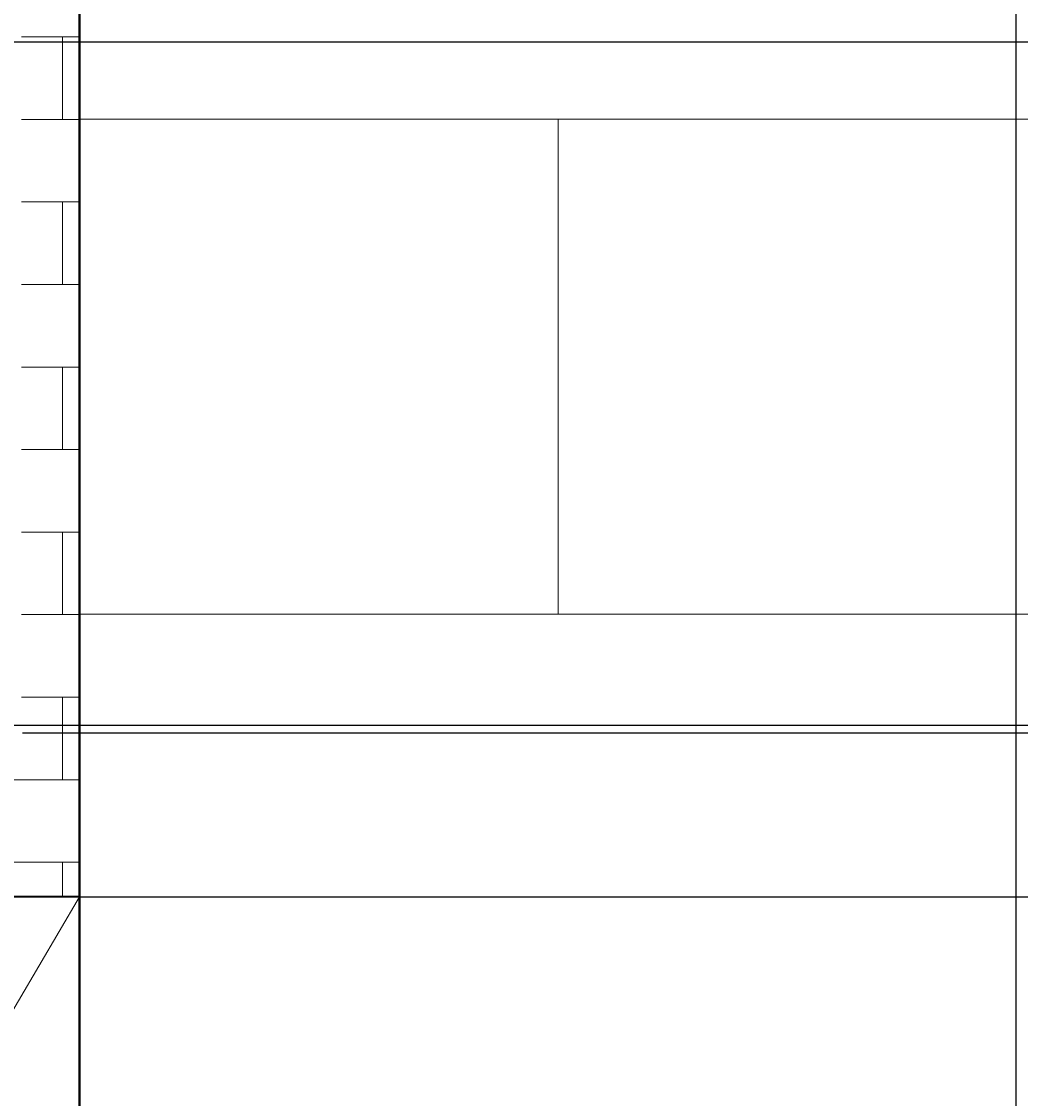
# Model space of a CAD drawing. Units: inches. Extents: x -26 to 776, y -22 to 650.
# Tile 19 of 62: x 285 to 358, y 145 to 223. Entities that reach past the tile are written whole.
import ezdxf

# ---------------------------------------------------------------- set-up
doc = ezdxf.new("R2010")
doc.units = ezdxf.units.IN
doc.header["$MEASUREMENT"] = 0
for name, color, linetype, lineweight in [('A-ANNO-DIMS', 2, 'Continuous', 18), ('A-WALL', 7, 'Continuous', 35), ('A-WALL-PATT', 8, 'Continuous', 13), ('A-WALL-TRIM', 7, 'Continuous', 18)]:
    doc.layers.add(name, color=color, linetype=linetype, lineweight=lineweight)
doc.styles.get("Standard").update_dxf_attribs({"font": 'arial.ttf'})
doc.dimstyles.get("Standard").update_dxf_attribs({"dimtxt": 0.5625, "dimasz": 0.18, "dimexe": 0.18, "dimexo": 0.0625, "dimgap": 0.09, "dimtad": 0, "dimtih": 1, "dimtoh": 1, "dimdec": 4, "dimzin": 0, "dimdsep": 46, "dimlunit": 4, "dimtxsty": 'Standard', "dimcen": 0.09, "dimadec": 0, "dimazin": 0, "dimtfac": 1, "dimtdec": 4, "dimtofl": 0, "dimtmove": 0, "dimatfit": 3, "dimfxl": 1, "dimtolj": 1, "dimtzin": 0, "dimarcsym": 0})

# ---------------------------------------------------------------- blocks, each defined once
blk = doc.blocks.new('*D26')
at = {"layer": 'A-ANNO-DIMS', "color": 0, "lineweight": -2, "transparency": 16777216}
for p, q in [((91.707, 171.973), (775.335, 171.973)), ((775.155, 171.793), (775.155, 166.105)), ((775.155, 159.662), (775.155, 165.351)), ((82.196, 159.482), (775.335, 159.482))]:
    blk.add_line(p, q, dxfattribs=at)
at = {"layer": 'A-ANNO-DIMS', "color": 0, "transparency": 16777216}
for points in [[(775.125, 171.793), (775.185, 171.793), (775.155, 171.973)], [(775.125, 159.662), (775.185, 159.662), (775.155, 159.482)]]:
    blk.add_solid(points, dxfattribs=at)
at = {"layer": 'Defpoints', "color": 0, "transparency": 16777216}
for p in [(91.645, 171.973), (775.155, 171.973), (82.134, 159.482)]:
    blk.add_point(p, dxfattribs=at)
at = {"layer": 'A-ANNO-DIMS', "color": 0, "transparency": 16777216, "insert": (775.155, 165.728), "char_height": 0.5625, "attachment_point": 5}
blk.add_mtext('\\A1;12.49', dxfattribs=at)
blk = doc.blocks.new('*D28')
at = {"layer": 'A-ANNO-DIMS', "color": 0, "lineweight": -2, "transparency": 16777216}
for p, q in [((285.08, 314.119), (775.335, 314.119)), ((775.155, 313.939), (775.155, 243.141)), ((775.155, 171.597), (775.155, 242.396)), ((285.08, 171.417), (775.335, 171.417))]:
    blk.add_line(p, q, dxfattribs=at)
at = {"layer": 'A-ANNO-DIMS', "color": 0, "transparency": 16777216}
for points in [[(775.125, 313.939), (775.185, 313.939), (775.155, 314.119)], [(775.125, 171.597), (775.185, 171.597), (775.155, 171.417)]]:
    blk.add_solid(points, dxfattribs=at)
at = {"layer": 'Defpoints', "color": 0, "transparency": 16777216}
for p in [(285.018, 314.119), (775.155, 314.119), (285.018, 171.417)]:
    blk.add_point(p, dxfattribs=at)
at = {"layer": 'A-ANNO-DIMS', "color": 0, "transparency": 16777216, "insert": (775.155, 242.768), "char_height": 0.5625, "attachment_point": 5}
blk.add_mtext('\\A1;142.7', dxfattribs=at)
blk = doc.blocks.new('*D34')
at = {"layer": 'A-ANNO-DIMS', "color": 0, "lineweight": -2, "transparency": 16777216}
for p, q in [((228.573, 528.296), (228.573, -21.315)), ((357.303, 528.361), (357.303, -21.315)), ((228.753, -21.135), (291.707, -21.135)), ((357.123, -21.135), (294.17, -21.135))]:
    blk.add_line(p, q, dxfattribs=at)
at = {"layer": 'A-ANNO-DIMS', "color": 0, "transparency": 16777216}
for points in [[(228.753, -21.105), (228.753, -21.165), (228.573, -21.135)], [(357.123, -21.105), (357.123, -21.165), (357.303, -21.135)]]:
    blk.add_solid(points, dxfattribs=at)
at = {"layer": 'Defpoints', "color": 0, "transparency": 16777216}
for p in [(357.303, 528.423), (228.573, 528.358), (357.303, -21.135)]:
    blk.add_point(p, dxfattribs=at)
at = {"layer": 'A-ANNO-DIMS', "color": 0, "transparency": 16777216, "insert": (292.938, -21.135), "char_height": 0.5625, "attachment_point": 5}
blk.add_mtext('\\A1;128.73', dxfattribs=at)
blk = doc.blocks.new('*D39')
at = {"layer": 'A-ANNO-DIMS', "color": 0, "lineweight": -2, "transparency": 16777216}
for p, q in [((289.242, 15.545), (289.242, 649.856)), ((425.743, 15.545), (425.743, 649.856)), ((289.422, 649.676), (356.478, 649.676)), ((425.563, 649.676), (358.508, 649.676))]:
    blk.add_line(p, q, dxfattribs=at)
at = {"layer": 'A-ANNO-DIMS', "color": 0, "transparency": 16777216}
for points in [[(289.422, 649.706), (289.422, 649.646), (289.242, 649.676)], [(425.563, 649.706), (425.563, 649.646), (425.743, 649.676)]]:
    blk.add_solid(points, dxfattribs=at)
at = {"layer": 'Defpoints', "color": 0, "transparency": 16777216}
for p in [(425.743, 649.676), (289.242, 15.482), (425.743, 15.482)]:
    blk.add_point(p, dxfattribs=at)
at = {"layer": 'A-ANNO-DIMS', "color": 0, "transparency": 16777216, "insert": (357.493, 649.676), "char_height": 0.5625, "attachment_point": 5}
blk.add_mtext('\\A1;136.5', dxfattribs=at)
blk = doc.blocks.new('*D41')
at = {"layer": 'A-ANNO-DIMS', "color": 0, "lineweight": -2, "transparency": 16777216}
for p, q in [((11.17, 221.641), (775.335, 221.641)), ((775.155, 221.461), (775.155, 190.939)), ((775.155, 159.662), (775.155, 190.185)), ((11.17, 159.482), (775.335, 159.482))]:
    blk.add_line(p, q, dxfattribs=at)
at = {"layer": 'A-ANNO-DIMS', "color": 0, "transparency": 16777216}
for points in [[(775.125, 221.461), (775.185, 221.461), (775.155, 221.641)], [(775.125, 159.662), (775.185, 159.662), (775.155, 159.482)]]:
    blk.add_solid(points, dxfattribs=at)
at = {"layer": 'Defpoints', "color": 0, "transparency": 16777216}
for p in [(11.107, 221.641), (775.155, 221.641), (11.107, 159.482)]:
    blk.add_point(p, dxfattribs=at)
at = {"layer": 'A-ANNO-DIMS', "color": 0, "transparency": 16777216, "insert": (775.155, 190.562), "char_height": 0.5625, "attachment_point": 5}
blk.add_mtext('\\A1;62.16', dxfattribs=at)
blk = doc.blocks.new('*D42')
at = {"layer": 'A-ANNO-DIMS', "color": 0, "lineweight": -2, "transparency": 16777216}
for p, q in [((285.08, 171.417), (775.335, 171.417)), ((775.155, 171.237), (775.155, 165.827)), ((775.155, 159.662), (775.155, 165.072)), ((289.305, 159.482), (775.335, 159.482))]:
    blk.add_line(p, q, dxfattribs=at)
at = {"layer": 'A-ANNO-DIMS', "color": 0, "transparency": 16777216}
for points in [[(775.125, 171.237), (775.185, 171.237), (775.155, 171.417)], [(775.125, 159.662), (775.185, 159.662), (775.155, 159.482)]]:
    blk.add_solid(points, dxfattribs=at)
at = {"layer": 'Defpoints', "color": 0, "transparency": 16777216}
for p in [(285.018, 171.417), (775.155, 171.417), (289.242, 159.482)]:
    blk.add_point(p, dxfattribs=at)
at = {"layer": 'A-ANNO-DIMS', "color": 0, "transparency": 16777216, "insert": (775.155, 165.45), "char_height": 0.5625, "attachment_point": 5}
blk.add_mtext('\\A1;11.935', dxfattribs=at)

msp = doc.modelspace()

# ---------------------------------------------------------------- hatches: boundary and pattern name
at = {"layer": 'A-WALL-PATT'}
h = msp.add_hatch(dxfattribs=at)
h.set_pattern_fill('AR-B816', color=256, scale=0.75)
h.paths.add_polyline_path([(289.2424, 504.4205), (231.4249, 504.4205), (231.4249, 458.1203), (231.4249, 221.6413), (231.4249, 209.6413), (231.4249, 159.4824), (285.0179, 159.4824), (285.0179, 171.4173), (236.4647, 171.4173), (236.4647, 294.4171), (236.4647, 303.3046), (285.0179, 303.3046), (285.0179, 294.4171), (285.0179, 171.4173), (285.0179, 159.4824), (289.2424, 159.4824), (289.2424, 291.1798), (289.2424, 458.1203)])
h.paths.add_polyline_path([(285.0179, 446.0063), (285.0179, 437.1188), (285.0179, 314.119), (236.4647, 314.119), (236.4647, 437.1188), (236.4647, 446.0063)], flags=16)
h = msp.add_hatch(dxfattribs=at)
h.set_pattern_fill('AR-B816', color=256, scale=4.5)
h.paths.add_polyline_path([(425.7434, 448.2114), (289.2424, 496.9554), (289.2424, 458.1203), (289.2424, 291.1798), (289.2424, 20.7937), (425.7434, 20.7937), (425.7434, 283.2492)])

# ---------------------------------------------------------------- linework, layer by layer
at = {"layer": 'A-WALL'}
for p, q in [((289.2424, 159.4824), (289.2424, 291.1798)), ((289.2424, 291.1798), (289.2424, 15.4824)), ((289.2424, 159.4824), (231.4249, 159.4824)), ((289.2424, 15.4824), (289.2424, 159.4824))]:
    msp.add_line(p, q, dxfattribs=at)
at = {"layer": 'A-WALL-TRIM'}
msp.add_line((280.6173, 144.8359), (289.2424, 159.4824), dxfattribs=at)

# ---------------------------------------------------------------- dimensions: what is measured, and where the dimension line sits
at = {"layer": 'A-ANNO-DIMS'}
for base, p1, p2, override, picture, middle in [((425.7434, 649.6763), (289.2424, 15.4824), (425.7434, 15.4824), {"dimdec": 1, "dimlfac": 1, "dimrnd": 0, "dimzin": 0, "dimdsep": 46, "dimlunit": 2}, '*D39', (357.4929, 649.6763)), ((357.3034, -21.1349), (228.5733, 528.3585), (357.3034, 528.4233), {"dimdec": 2, "dimlfac": 1, "dimrnd": 0, "dimzin": 0, "dimdsep": 46, "dimlunit": 2}, '*D34', (292.9384, -21.1349))]:
    dim = msp.add_linear_dim(base=base, p1=p1, p2=p2, dimstyle='Standard', override=override, dxfattribs=at)
    dim.commit()
    dim.dimension.update_dxf_attribs({"geometry": picture, "text_midpoint": middle})
for base, p1, p2, override, picture, middle in [((775.1553, 314.119), (285.0179, 171.4173), (285.0179, 314.119), {"dimdec": 1, "dimlfac": 1, "dimrnd": 0, "dimzin": 0, "dimdsep": 46, "dimlunit": 2}, '*D28', (775.1553, 242.7682)), ((775.1553, 221.6413), (11.1074, 159.4824), (11.1074, 221.6413), {"dimdec": 2, "dimlfac": 1, "dimrnd": 0, "dimzin": 0, "dimdsep": 46, "dimlunit": 2}, '*D41', (775.1553, 190.5618)), ((775.1553, 171.9734), (82.134, 159.4824), (91.6448, 171.9734), {"dimdec": 2, "dimlfac": 1, "dimrnd": 0, "dimzin": 0, "dimdsep": 46, "dimlunit": 2}, '*D26', (775.1553, 165.7279)), ((775.1553, 171.4173), (289.2424, 159.4824), (285.0179, 171.4173), {"dimdec": 3, "dimlfac": 1, "dimrnd": 0, "dimzin": 0, "dimdsep": 46, "dimlunit": 2}, '*D42', (775.1553, 165.4498))]:
    dim = msp.add_linear_dim(base=base, p1=p1, p2=p2, angle=90, dimstyle='Standard', override=override, dxfattribs=at)
    dim.commit()
    dim.dimension.update_dxf_attribs({"geometry": picture, "text_midpoint": middle})

doc.saveas('drawing.dxf')
